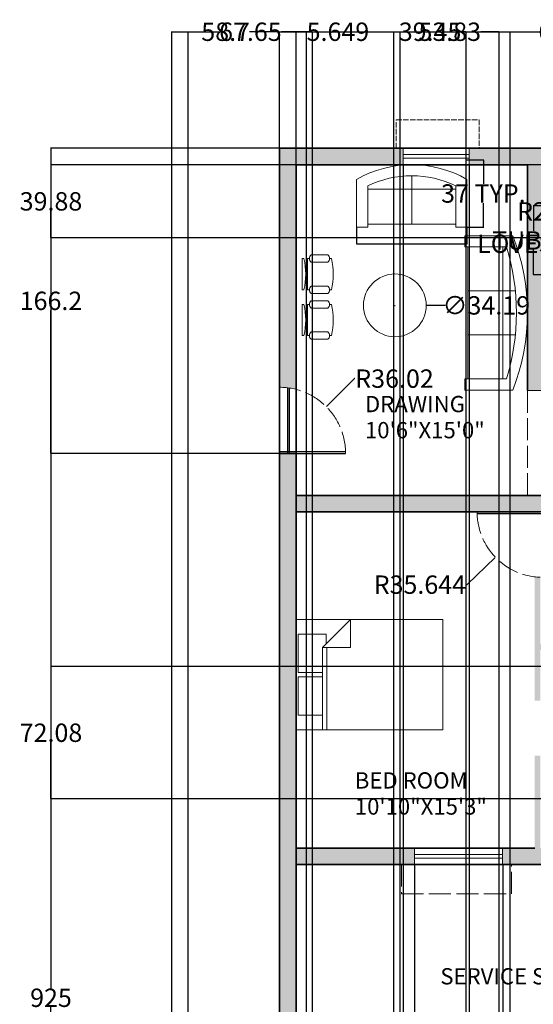
# Model space of a CAD drawing. Units: inches. Extents: x 300 to 1007, y 2 to 1069.
# Tile 8 of 12: x 337 to 617, y 533 to 1069. Entities that reach past the tile are written whole.
import ezdxf

# ---------------------------------------------------------------- set-up
doc = ezdxf.new("R2010")
doc.units = ezdxf.units.IN
doc.header["$MEASUREMENT"] = 0
doc.linetypes.add('ACAD_ISO02W100', pattern=[15, 12, -3])
for name, color, linetype, lineweight in [('A-ANNO-DIMS', 2, 'Continuous', 18), ('A-ANNO-TEXT', 7, 'Continuous', 18), ('A-AREA-IDEN', 7, 'Continuous', 18), ('A-DOOR', 3, 'Continuous', 25), ('A-DOOR-SWNG', 3, 'ACAD_ISO02W100', 13), ('A-FLOR-SLAB', 7, 'Continuous', 35), ('A-FURN', 8, 'Continuous', 18), ('A-GLAZ', 4, 'Continuous', 18), ('A-GLAZ-OVHD', 8, 'ACAD_ISO02W100', 13), ('A-WALL', 7, 'Continuous', 35), ('A-WALL-OVHD', 8, 'ACAD_ISO02W100', 18)]:
    doc.layers.add(name, color=color, linetype=linetype, lineweight=lineweight)
doc.layers.add('A-WALL-PATT', color=9, linetype='Continuous', lineweight=9, true_color=0xc7c8ca)
doc.styles.get("Standard").update_dxf_attribs({"font": 'arial.ttf'})
doc.dimstyles.get("Standard").update_dxf_attribs({"dimtxt": 10, "dimasz": 0.18, "dimexe": 0.18, "dimexo": 0.0625, "dimgap": 0.09, "dimtad": 0, "dimtih": 1, "dimtoh": 1, "dimdec": 0, "dimzin": 0, "dimdsep": 46, "dimlunit": 3, "dimtxsty": 'Standard', "dimcen": 0.09, "dimadec": 0, "dimazin": 0, "dimtfac": 1, "dimtdec": 0, "dimtofl": 0, "dimtmove": 0, "dimatfit": 3, "dimfxl": 1, "dimtolj": 1, "dimtzin": 0, "dimarcsym": 0})

# ---------------------------------------------------------------- blocks, each defined once
blk = doc.blocks.new('Chair - Desk')
for p, q in [((-8.5, 0), (-8.5, -1)), ((-8.5, 0), (8.5, 0)), ((8.5, 0), (8.5, -1)), ((-10.5, -5), (-10.5, -14)), ((-8.5, -3), (-8.5, -4)), ((-8.5, -3), (8.5, -3)), ((-6.5, -14), (-6.5, -5)), ((-2, -3), (-2, -1.9355)), ((2, -1.9576), (2, -3)), ((6.5, -5), (6.5, -14)), ((8.5, -3), (8.5, -4)), ((10.5, -14), (10.5, -5)), ((-8.5, -15), (-8.5, -16)), ((8.5, -15), (8.5, -16))]:
    blk.add_line(p, q)
for centre, radius, start, end in [((-8.5, -6.5), 2.5, 36.8699, 143.1301), ((0, 34.625), 36.625, 256.5803, 283.4197), ((8.5, -6.5), 2.5, 36.8699, 143.1301), ((-8.5, -12.5), 2.5, 216.8699, 323.1301), ((0, 19.625), 36.625, 256.5803, 283.4197), ((8.5, -12.5), 2.5, 216.8699, 323.1301)]:
    blk.add_arc(centre, radius, start, end)
blk = doc.blocks.new('Sofa - Roundback 7 ft.')
for p, q in [((-12.00002, -32.4421), (-12.00003, -6.5971)), ((11.99997, -32.4421), (11.99998, -6.5971)), ((-36.000027, -34), (-36.000027, -11.4696)), ((-35.999844, -13.3819), (35.9998, -13.3819)), ((35.99998, -34), (35.99998, -11.4696)), ((-36.000027, -32.4421), (35.99998, -32.4421))]:
    blk.add_line(p, q)
for points in [[(-36.000027, -34), (-42.000027, -34), (-42.000027, -8)], [(41.99998, -8), (41.99998, -34), (35.99998, -34)]]:
    blk.add_lwpolyline(points)
for centre, radius, start, end in [((0, -114.25), 114.25, 68.43141, 111.5686), ((-0.00001, -127.1968), 121.1968, 72.72033, 107.2797)]:
    blk.add_arc(centre, radius, start, end)
blk = doc.blocks.new('Sofa - Roundback Loveseat 5 ft.')
for p, q in [((0, -32.44198), (0, -5.99998)), ((-24, -33.99998), (-24, -11.46958)), ((-23.9998, -13.38178), (23.99986, -13.38178)), ((24.00004, -33.99998), (24.00004, -11.46958)), ((-24, -32.44198), (24.00004, -32.44198))]:
    blk.add_line(p, q)
for points in [[(-24, -33.99998), (-30, -33.99998), (-30, -7.99998)], [(30.00004, -7.99998), (30.00004, -33.99998), (24.00004, -33.99998)]]:
    blk.add_lwpolyline(points)
for centre, radius, start, end in [((0, -60.24998), 60.24998, 60.13715, 119.8628), ((0, -61.38438), 55.38444, 64.32083, 115.6792)]:
    blk.add_arc(centre, radius, start, end)
blk = doc.blocks.new('Bed - Queen')
for p, q in [((0, -80.00003), (0, 0)), ((0, 0), (59.99999, 0)), ((59.99999, 0), (59.99999, -80.00003)), ((7.99999, -1.2), (28.79998, -1.2)), ((7.99999, -14.4), (7.99999, -1.2)), ((28.79998, -1.2), (28.79998, -14.4)), ((31.19999, -1.2), (51.99999, -1.2)), ((31.19999, -14.4), (31.19999, -1.2)), ((51.99999, -1.2), (51.99999, -16.4)), ((0, -14.4), (44.8, -14.4)), ((59.99999, -29.6), (44.8, -14.4)), ((44.8, -14.4), (44.8, -29.6)), ((44.8, -16.8), (0, -16.8)), ((51.99999, -16.4), (46.79936, -16.4)), ((44.8, -29.6), (59.99999, -29.6)), ((59.99999, -80.00003), (0, -80.00003))]:
    blk.add_line(p, q)
blk = doc.blocks.new('WIN-48')
for p, q in [((-47.83, 0), (-47.83, 4.5)), ((-47.83, 4.5), (-47.83, -4.5)), ((0, 1), (-47.83, 1)), ((0, 4.5), (0, -4.5)), ((0, -1), (-47.83, -1))]:
    blk.add_line(p, q)
blk = doc.blocks.new('WIN-36')
for p, q in [((-36, -4.5), (-36, 4.5)), ((0, 1), (-36, 1)), ((-36, 0), (-36, -4.5)), ((0, -4.5), (0, 4.5)), ((0, -1), (-36, -1))]:
    blk.add_line(p, q)
blk = doc.blocks.new('WINDOW-HOOD-45')
at = {"ltscale": 0.25}
for p, q in [((0, 0), (0, 15.48)), ((0, 15.48), (45.18, 15.48)), ((45.18, 15.48), (45.18, 0))]:
    blk.add_line(p, q, dxfattribs=at)
blk = doc.blocks.new('*D39')
at = {"layer": 'A-ANNO-DIMS', "color": 0, "lineweight": -2, "transparency": 16777216}
for p, q in [((622.76, 968.04), (617.01, 968.04)), ((617.19, 967.86), (617.19, 954.44)), ((617.19, 930.63), (617.19, 944.04)), ((622.76, 930.45), (617.01, 930.45))]:
    blk.add_line(p, q, dxfattribs=at)
at = {"layer": 'A-ANNO-DIMS', "color": 0, "transparency": 16777216}
for points in [[(617.16, 967.86), (617.22, 967.86), (617.19, 968.04)], [(617.16, 930.63), (617.22, 930.63), (617.19, 930.45)]]:
    blk.add_solid(points, dxfattribs=at)
at = {"layer": 'Defpoints', "color": 0, "transparency": 16777216}
for p in [(622.83, 968.04), (617.19, 930.45), (622.83, 930.45)]:
    blk.add_point(p, dxfattribs=at)
at = {"layer": 'A-ANNO-DIMS', "color": 0, "transparency": 16777216, "insert": (617.19, 949.24), "char_height": 10, "attachment_point": 5}
blk.add_mtext('\\A1;TUB 38', dxfattribs=at)
blk = doc.blocks.new('*D49')
at = {"layer": 'A-ANNO-DIMS', "color": 0, "lineweight": -2, "transparency": 16777216}
for p, q in [((520.83, 956.38), (520.83, 947.27)), ((580.83, 956.38), (580.83, 947.27)), ((521.01, 947.45), (580.65, 947.45)), ((580.83, 947.45), (581.01, 947.45))]:
    blk.add_line(p, q, dxfattribs=at)
at = {"layer": 'A-ANNO-DIMS', "color": 0, "transparency": 16777216}
for points in [[(521.01, 947.48), (521.01, 947.42), (520.83, 947.45)], [(580.65, 947.48), (580.65, 947.42), (580.83, 947.45)]]:
    blk.add_solid(points, dxfattribs=at)
at = {"layer": 'Defpoints', "color": 0, "transparency": 16777216}
for p in [(520.83, 956.45), (580.83, 956.45), (580.83, 947.45)]:
    blk.add_point(p, dxfattribs=at)
at = {"layer": 'A-ANNO-DIMS', "color": 0, "transparency": 16777216, "insert": (644.03, 947.45), "char_height": 10, "attachment_point": 5}
blk.add_mtext('\\A1;LOVESEAT 60 TYP.', dxfattribs=at)
blk = doc.blocks.new('*D50')
at = {"layer": 'A-ANNO-DIMS', "color": 0, "lineweight": -2, "transparency": 16777216}
for p, q in [((580.89, 993.11), (590.01, 993.11)), ((589.83, 992.93), (589.83, 979.98)), ((589.83, 956.63), (589.83, 969.58)), ((580.89, 956.45), (590.01, 956.45))]:
    blk.add_line(p, q, dxfattribs=at)
at = {"layer": 'A-ANNO-DIMS', "color": 0, "transparency": 16777216}
for points in [[(589.8, 992.93), (589.86, 992.93), (589.83, 993.11)], [(589.8, 956.63), (589.86, 956.63), (589.83, 956.45)]]:
    blk.add_solid(points, dxfattribs=at)
at = {"layer": 'Defpoints', "color": 0, "transparency": 16777216}
for p in [(580.83, 993.11), (589.83, 993.11), (580.83, 956.45)]:
    blk.add_point(p, dxfattribs=at)
at = {"layer": 'A-ANNO-DIMS', "color": 0, "transparency": 16777216, "insert": (589.83, 974.78), "char_height": 10, "attachment_point": 5}
blk.add_mtext('\\A1;37 TYP.', dxfattribs=at)
blk = doc.blocks.new('*D74')
at = {"layer": 'A-ANNO-DIMS', "color": 0, "lineweight": -2, "transparency": 16777216}
for p, q in [((478.76, 999.45), (354.19, 999.45)), ((354.37, 999.27), (354.37, 542.11)), ((354.37, 74.56), (354.37, 531.72)), ((420.06, 74.38), (354.19, 74.38))]:
    blk.add_line(p, q, dxfattribs=at)
at = {"layer": 'A-ANNO-DIMS', "color": 0, "transparency": 16777216}
for points in [[(354.34, 999.27), (354.4, 999.27), (354.37, 999.45)], [(354.34, 74.56), (354.4, 74.56), (354.37, 74.38)]]:
    blk.add_solid(points, dxfattribs=at)
at = {"layer": 'Defpoints', "color": 0, "transparency": 16777216}
for p in [(354.37, 999.45), (478.83, 999.45), (420.12, 74.38)]:
    blk.add_point(p, dxfattribs=at)
at = {"layer": 'A-ANNO-DIMS', "color": 0, "transparency": 16777216, "insert": (354.37, 536.92), "char_height": 10, "attachment_point": 5}
blk.add_mtext('\\A1;925', dxfattribs=at)
blk = doc.blocks.new('*D75')
at = {"layer": 'A-ANNO-DIMS', "color": 0, "lineweight": -2, "transparency": 16777216}
for p, q in [((478.83, 999.51), (478.83, 1063.03)), ((479.01, 1062.85), (653.74, 1062.85)), ((850.65, 1062.85), (675.91, 1062.85)), ((850.83, 999.51), (850.83, 1063.03))]:
    blk.add_line(p, q, dxfattribs=at)
at = {"layer": 'A-ANNO-DIMS', "color": 0, "transparency": 16777216}
for points in [[(479.01, 1062.88), (479.01, 1062.82), (478.83, 1062.85)], [(850.65, 1062.88), (850.65, 1062.82), (850.83, 1062.85)]]:
    blk.add_solid(points, dxfattribs=at)
at = {"layer": 'Defpoints', "color": 0, "transparency": 16777216}
for p in [(850.83, 1062.85), (478.83, 999.45), (850.83, 999.45)]:
    blk.add_point(p, dxfattribs=at)
at = {"layer": 'A-ANNO-DIMS', "color": 0, "transparency": 16777216, "insert": (664.83, 1062.85), "char_height": 10, "attachment_point": 5}
blk.add_mtext('\\A1;372', dxfattribs=at)
blk = doc.blocks.new('*D79')
at = {"layer": 'A-ANNO-DIMS', "color": 0, "lineweight": -2, "transparency": 16777216}
for p, q in [((420.12, 482.45), (420.12, 1063.03)), ((420.3, 1062.85), (436.4, 1062.85)), ((478.65, 1062.85), (462.55, 1062.85)), ((478.83, 482.45), (478.83, 1063.03))]:
    blk.add_line(p, q, dxfattribs=at)
at = {"layer": 'A-ANNO-DIMS', "color": 0, "transparency": 16777216}
for points in [[(420.3, 1062.88), (420.3, 1062.82), (420.12, 1062.85)], [(478.65, 1062.88), (478.65, 1062.82), (478.83, 1062.85)]]:
    blk.add_solid(points, dxfattribs=at)
at = {"layer": 'Defpoints', "color": 0, "transparency": 16777216}
for p in [(478.83, 1062.85), (420.12, 482.38), (478.83, 482.38)]:
    blk.add_point(p, dxfattribs=at)
at = {"layer": 'A-ANNO-DIMS', "color": 0, "transparency": 16777216, "insert": (449.47, 1062.85), "char_height": 10, "attachment_point": 5}
blk.add_mtext('\\A1;58.7', dxfattribs=at)
blk = doc.blocks.new('*D81')
at = {"layer": 'A-ANNO-DIMS', "color": 0, "lineweight": -2, "transparency": 16777216}
for p, q in [((705.53, 717.25), (354.19, 717.25)), ((354.37, 717.07), (354.37, 686.41)), ((354.37, 645.35), (354.37, 676.01)), ((705.53, 645.17), (354.19, 645.17))]:
    blk.add_line(p, q, dxfattribs=at)
at = {"layer": 'A-ANNO-DIMS', "color": 0, "transparency": 16777216}
for points in [[(354.34, 717.07), (354.4, 717.07), (354.37, 717.25)], [(354.34, 645.35), (354.4, 645.35), (354.37, 645.17)]]:
    blk.add_solid(points, dxfattribs=at)
at = {"layer": 'Defpoints', "color": 0, "transparency": 16777216}
for p in [(354.37, 717.25), (705.59, 717.25), (705.59, 645.17)]:
    blk.add_point(p, dxfattribs=at)
at = {"layer": 'A-ANNO-DIMS', "color": 0, "transparency": 16777216, "insert": (354.37, 681.21), "char_height": 10, "attachment_point": 5}
blk.add_mtext('\\A1;72.08', dxfattribs=at)
blk = doc.blocks.new('*D88')
at = {"layer": 'A-ANNO-DIMS', "color": 0, "lineweight": -2, "transparency": 16777216}
for p, q in [((429.12, 83.45), (429.12, 1063.03)), ((429.3, 1062.85), (445.92, 1062.85)), ((496.59, 1062.85), (479.97, 1062.85)), ((496.77, 83.45), (496.77, 1063.03))]:
    blk.add_line(p, q, dxfattribs=at)
at = {"layer": 'A-ANNO-DIMS', "color": 0, "transparency": 16777216}
for points in [[(429.3, 1062.88), (429.3, 1062.82), (429.12, 1062.85)], [(496.59, 1062.88), (496.59, 1062.82), (496.77, 1062.85)]]:
    blk.add_solid(points, dxfattribs=at)
at = {"layer": 'Defpoints', "color": 0, "transparency": 16777216}
for p in [(496.77, 1062.85), (429.12, 83.38), (496.77, 83.38)]:
    blk.add_point(p, dxfattribs=at)
at = {"layer": 'A-ANNO-DIMS', "color": 0, "transparency": 16777216, "insert": (462.95, 1062.85), "char_height": 10, "attachment_point": 5}
blk.add_mtext('\\A1;67.65', dxfattribs=at)
blk = doc.blocks.new('*D89')
at = {"layer": 'A-ANNO-DIMS', "color": 0, "lineweight": -2, "transparency": 16777216}
for p, q in [((544.6, 83.45), (544.6, 1063.03)), ((544.78, 1062.85), (554.56, 1062.85)), ((598.25, 1062.85), (588.48, 1062.85)), ((598.43, 83.45), (598.43, 1063.03))]:
    blk.add_line(p, q, dxfattribs=at)
at = {"layer": 'A-ANNO-DIMS', "color": 0, "transparency": 16777216}
for points in [[(544.78, 1062.88), (544.78, 1062.82), (544.6, 1062.85)], [(598.25, 1062.88), (598.25, 1062.82), (598.43, 1062.85)]]:
    blk.add_solid(points, dxfattribs=at)
at = {"layer": 'Defpoints', "color": 0, "transparency": 16777216}
for p in [(598.43, 1062.85), (544.6, 83.38), (598.43, 83.38)]:
    blk.add_point(p, dxfattribs=at)
at = {"layer": 'A-ANNO-DIMS', "color": 0, "transparency": 16777216, "insert": (571.52, 1062.85), "char_height": 10, "attachment_point": 5}
blk.add_mtext('\\A1;53.83', dxfattribs=at)
blk = doc.blocks.new('*D93')
at = {"layer": 'A-ANNO-DIMS', "color": 0, "lineweight": -2, "transparency": 16777216}
for p, q in [((478.76, 999.45), (354.19, 999.45)), ((354.37, 999.27), (354.37, 921.55)), ((354.37, 833.44), (354.37, 911.16)), ((478.76, 833.26), (354.19, 833.26))]:
    blk.add_line(p, q, dxfattribs=at)
at = {"layer": 'A-ANNO-DIMS', "color": 0, "transparency": 16777216}
for points in [[(354.34, 999.27), (354.4, 999.27), (354.37, 999.45)], [(354.34, 833.44), (354.4, 833.44), (354.37, 833.26)]]:
    blk.add_solid(points, dxfattribs=at)
at = {"layer": 'Defpoints', "color": 0, "transparency": 16777216}
for p in [(354.37, 999.45), (478.83, 999.45), (478.83, 833.26)]:
    blk.add_point(p, dxfattribs=at)
at = {"layer": 'A-ANNO-DIMS', "color": 0, "transparency": 16777216, "insert": (354.37, 916.35), "char_height": 10, "attachment_point": 5}
blk.add_mtext('\\A1;166.2', dxfattribs=at)
blk = doc.blocks.new('*D94')
at = {"layer": 'A-ANNO-DIMS', "color": 0, "lineweight": -2, "transparency": 16777216}
for p, q in [((841.76, 990.45), (354.19, 990.45)), ((354.37, 990.27), (354.37, 975.71)), ((354.37, 950.75), (354.37, 965.31)), ((841.76, 950.57), (354.19, 950.57))]:
    blk.add_line(p, q, dxfattribs=at)
at = {"layer": 'A-ANNO-DIMS', "color": 0, "transparency": 16777216}
for points in [[(354.34, 990.27), (354.4, 990.27), (354.37, 990.45)], [(354.34, 950.75), (354.4, 950.75), (354.37, 950.57)]]:
    blk.add_solid(points, dxfattribs=at)
at = {"layer": 'Defpoints', "color": 0, "transparency": 16777216}
for p in [(354.37, 990.45), (841.83, 990.45), (841.83, 950.57)]:
    blk.add_point(p, dxfattribs=at)
at = {"layer": 'A-ANNO-DIMS', "color": 0, "transparency": 16777216, "insert": (354.37, 970.51), "char_height": 10, "attachment_point": 5}
blk.add_mtext('\\A1;39.88', dxfattribs=at)
blk = doc.blocks.new('*D97')
at = {"layer": 'A-ANNO-DIMS', "color": 0, "lineweight": -2, "transparency": 16777216}
for p, q in [((487.83, 482.45), (487.83, 1063.03)), ((488.01, 1062.85), (493.3, 1062.85)), ((493.48, 482.45), (493.48, 1063.03)), ((493.48, 1062.85), (493.66, 1062.85))]:
    blk.add_line(p, q, dxfattribs=at)
at = {"layer": 'A-ANNO-DIMS', "color": 0, "transparency": 16777216}
for points in [[(488.01, 1062.88), (488.01, 1062.82), (487.83, 1062.85)], [(493.3, 1062.88), (493.3, 1062.82), (493.48, 1062.85)]]:
    blk.add_solid(points, dxfattribs=at)
at = {"layer": 'Defpoints', "color": 0, "transparency": 16777216}
for p in [(493.48, 1062.85), (487.83, 482.38), (493.48, 482.38)]:
    blk.add_point(p, dxfattribs=at)
at = {"layer": 'A-ANNO-DIMS', "color": 0, "transparency": 16777216, "insert": (510.63, 1062.85), "char_height": 10, "attachment_point": 5}
blk.add_mtext('\\A1;5.649', dxfattribs=at)
blk = doc.blocks.new('*D98')
at = {"layer": 'A-ANNO-DIMS', "color": 0, "lineweight": -2, "transparency": 16777216}
for p, q in [((541.08, 482.45), (541.08, 1063.03)), ((541.26, 1062.85), (543.81, 1062.85)), ((580.35, 1062.85), (577.8, 1062.85)), ((580.53, 482.45), (580.53, 1063.03))]:
    blk.add_line(p, q, dxfattribs=at)
at = {"layer": 'A-ANNO-DIMS', "color": 0, "transparency": 16777216}
for points in [[(541.26, 1062.88), (541.26, 1062.82), (541.08, 1062.85)], [(580.35, 1062.88), (580.35, 1062.82), (580.53, 1062.85)]]:
    blk.add_solid(points, dxfattribs=at)
at = {"layer": 'Defpoints', "color": 0, "transparency": 16777216}
for p in [(580.53, 1062.85), (541.08, 482.38), (580.53, 482.38)]:
    blk.add_point(p, dxfattribs=at)
at = {"layer": 'A-ANNO-DIMS', "color": 0, "transparency": 16777216, "insert": (560.81, 1062.85), "char_height": 10, "attachment_point": 5}
blk.add_mtext('\\A1;39.45', dxfattribs=at)
blk = doc.blocks.new('*D99')
at = {"layer": 'A-ANNO-DIMS', "color": 0, "lineweight": -2, "transparency": 16777216}
for p, q in [((604.49, 482.45), (604.49, 1063.03)), ((604.67, 1062.85), (619.83, 1062.85)), ((668.97, 1062.85), (653.8, 1062.85)), ((669.15, 482.45), (669.15, 1063.03))]:
    blk.add_line(p, q, dxfattribs=at)
at = {"layer": 'A-ANNO-DIMS', "color": 0, "transparency": 16777216}
for points in [[(604.67, 1062.88), (604.67, 1062.82), (604.49, 1062.85)], [(668.97, 1062.88), (668.97, 1062.82), (669.15, 1062.85)]]:
    blk.add_solid(points, dxfattribs=at)
at = {"layer": 'Defpoints', "color": 0, "transparency": 16777216}
for p in [(669.15, 1062.85), (604.49, 482.38), (669.15, 482.38)]:
    blk.add_point(p, dxfattribs=at)
at = {"layer": 'A-ANNO-DIMS', "color": 0, "transparency": 16777216, "insert": (636.82, 1062.85), "char_height": 10, "attachment_point": 5}
blk.add_mtext('\\A1;64.66', dxfattribs=at)
blk = doc.blocks.new('*D101')
at = {"layer": 'A-ANNO-DIMS', "color": 0, "lineweight": -2, "transparency": 16777216}
for p, q in [((487.83, 609.38), (487.83, 8.45)), ((552.34, 609.38), (552.34, 8.45)), ((488.01, 8.63), (504.06, 8.63)), ((552.16, 8.63), (536.11, 8.63))]:
    blk.add_line(p, q, dxfattribs=at)
at = {"layer": 'A-ANNO-DIMS', "color": 0, "transparency": 16777216}
for points in [[(488.01, 8.66), (488.01, 8.6), (487.83, 8.63)], [(552.16, 8.66), (552.16, 8.6), (552.34, 8.63)]]:
    blk.add_solid(points, dxfattribs=at)
at = {"layer": 'Defpoints', "color": 0, "transparency": 16777216}
for p in [(487.83, 609.45), (552.34, 609.45), (552.34, 8.63)]:
    blk.add_point(p, dxfattribs=at)
at = {"layer": 'A-ANNO-DIMS', "color": 0, "transparency": 16777216, "insert": (520.08, 8.63), "char_height": 10, "attachment_point": 5}
blk.add_mtext('\\A1;64.51', dxfattribs=at)
blk = doc.blocks.new('*D102')
at = {"layer": 'A-ANNO-DIMS', "color": 0, "lineweight": -2, "transparency": 16777216}
for p, q in [((600.34, 609.38), (600.34, 8.45)), ((652.99, 609.38), (652.99, 8.45)), ((600.52, 8.63), (609.71, 8.63)), ((652.81, 8.63), (643.62, 8.63))]:
    blk.add_line(p, q, dxfattribs=at)
at = {"layer": 'A-ANNO-DIMS', "color": 0, "transparency": 16777216}
for points in [[(600.52, 8.66), (600.52, 8.6), (600.34, 8.63)], [(652.81, 8.66), (652.81, 8.6), (652.99, 8.63)]]:
    blk.add_solid(points, dxfattribs=at)
at = {"layer": 'Defpoints', "color": 0, "transparency": 16777216}
for p in [(600.34, 609.45), (652.99, 609.45), (652.99, 8.63)]:
    blk.add_point(p, dxfattribs=at)
at = {"layer": 'A-ANNO-DIMS', "color": 0, "transparency": 16777216, "insert": (626.66, 8.63), "char_height": 10, "attachment_point": 5}
blk.add_mtext('\\A1;52.66', dxfattribs=at)
blk = doc.blocks.new('*D105')
at = {"layer": 'A-ANNO-DIMS', "color": 0, "lineweight": -2, "transparency": 16777216}
for p, q in [((487.83, 990.38), (487.83, 8.45)), ((546.1, 990.38), (546.1, 8.45)), ((488.01, 8.63), (499.99, 8.63)), ((545.92, 8.63), (533.94, 8.63))]:
    blk.add_line(p, q, dxfattribs=at)
at = {"layer": 'A-ANNO-DIMS', "color": 0, "transparency": 16777216}
for points in [[(488.01, 8.66), (488.01, 8.6), (487.83, 8.63)], [(545.92, 8.66), (545.92, 8.6), (546.1, 8.63)]]:
    blk.add_solid(points, dxfattribs=at)
at = {"layer": 'Defpoints', "color": 0, "transparency": 16777216}
for p in [(487.83, 990.45), (546.1, 990.45), (546.1, 8.63)]:
    blk.add_point(p, dxfattribs=at)
at = {"layer": 'A-ANNO-DIMS', "color": 0, "transparency": 16777216, "insert": (516.97, 8.63), "char_height": 10, "attachment_point": 5}
blk.add_mtext('\\A1;58.28', dxfattribs=at)
blk = doc.blocks.new('*D106')
at = {"layer": 'A-ANNO-DIMS', "color": 0, "lineweight": -2, "transparency": 16777216}
for p, q in [((582.11, 990.38), (582.11, 8.45)), ((630.49, 990.38), (630.49, 8.45)), ((582.29, 8.63), (589.12, 8.63)), ((630.31, 8.63), (623.47, 8.63))]:
    blk.add_line(p, q, dxfattribs=at)
at = {"layer": 'A-ANNO-DIMS', "color": 0, "transparency": 16777216}
for points in [[(582.29, 8.66), (582.29, 8.6), (582.11, 8.63)], [(630.31, 8.66), (630.31, 8.6), (630.49, 8.63)]]:
    blk.add_solid(points, dxfattribs=at)
at = {"layer": 'Defpoints', "color": 0, "transparency": 16777216}
for p in [(582.11, 990.45), (630.49, 990.45), (630.49, 8.63)]:
    blk.add_point(p, dxfattribs=at)
at = {"layer": 'A-ANNO-DIMS', "color": 0, "transparency": 16777216, "insert": (606.3, 8.63), "char_height": 10, "attachment_point": 5}
blk.add_mtext('\\A1;48.38', dxfattribs=at)
blk = doc.blocks.new('*D110')
at = {"layer": 'A-ANNO-DIMS', "color": 0, "lineweight": -2, "transparency": 16777216}
for p, q in [((541.56, 913.87), (541.74, 913.87)), ((541.65, 913.78), (541.65, 913.96)), ((569, 913.87), (558.92, 913.87))]:
    blk.add_line(p, q, dxfattribs=at)
at = {"layer": 'A-ANNO-DIMS', "color": 0, "transparency": 16777216}
blk.add_solid([(558.92, 913.9), (558.92, 913.84), (558.74, 913.87)], dxfattribs=at)
at = {"layer": 'Defpoints', "color": 0, "transparency": 16777216}
for p in [(524.55, 913.87), (558.74, 913.87)]:
    blk.add_point(p, dxfattribs=at)
at = {"layer": 'A-ANNO-DIMS', "color": 0, "transparency": 16777216, "insert": (591.41, 913.87), "char_height": 10, "attachment_point": 5}
blk.add_mtext('\\A1;∅34.19', dxfattribs=at)
blk = doc.blocks.new('*D112')
at = {"layer": 'A-ANNO-DIMS', "color": 0, "lineweight": -2, "transparency": 16777216}
for p, q in [((519.57, 874), (504.41, 858.85)), ((519.75, 874), (519.57, 874)), ((478.72, 833.26), (478.9, 833.26)), ((478.81, 833.17), (478.81, 833.35))]:
    blk.add_line(p, q, dxfattribs=at)
at = {"layer": 'A-ANNO-DIMS', "color": 0, "transparency": 16777216}
blk.add_solid([(504.39, 858.87), (504.43, 858.83), (504.28, 858.72)], dxfattribs=at)
at = {"layer": 'Defpoints', "color": 0, "transparency": 16777216}
for p in [(504.28, 858.72), (478.81, 833.26)]:
    blk.add_point(p, dxfattribs=at)
at = {"layer": 'A-ANNO-DIMS', "color": 0, "transparency": 16777216, "insert": (541.44, 874), "char_height": 10, "attachment_point": 5}
blk.add_mtext('\\A1;R36.02', dxfattribs=at)
blk = doc.blocks.new('*D113')
at = {"layer": 'A-ANNO-DIMS', "color": 0, "lineweight": -2, "transparency": 16777216}
for p, q in [((621.98, 801.45), (622.16, 801.45)), ((622.07, 801.36), (622.07, 801.54)), ((581.05, 761.83), (596.3, 776.56)), ((580.87, 761.83), (581.05, 761.83))]:
    blk.add_line(p, q, dxfattribs=at)
at = {"layer": 'A-ANNO-DIMS', "color": 0, "transparency": 16777216}
blk.add_solid([(596.28, 776.58), (596.32, 776.54), (596.43, 776.68)], dxfattribs=at)
at = {"layer": 'Defpoints', "color": 0, "transparency": 16777216}
for p in [(622.07, 801.45), (596.43, 776.68)]:
    blk.add_point(p, dxfattribs=at)
at = {"layer": 'A-ANNO-DIMS', "color": 0, "transparency": 16777216, "insert": (555.25, 761.83), "char_height": 10, "attachment_point": 5}
blk.add_mtext('\\A1;R35.644', dxfattribs=at)
blk = doc.blocks.new('*D118')
at = {"layer": 'A-ANNO-DIMS', "color": 0, "lineweight": -2, "transparency": 16777216}
for p, q in [((651.31, 965.03), (651.49, 965.03)), ((651.49, 965.03), (663.55, 952.19)), ((683.9, 930.45), (684.08, 930.45)), ((683.99, 930.36), (683.99, 930.54))]:
    blk.add_line(p, q, dxfattribs=at)
at = {"layer": 'A-ANNO-DIMS', "color": 0, "transparency": 16777216}
blk.add_solid([(663.57, 952.21), (663.53, 952.17), (663.68, 952.06)], dxfattribs=at)
at = {"layer": 'Defpoints', "color": 0, "transparency": 16777216}
for p in [(663.68, 952.06), (683.99, 930.45)]:
    blk.add_point(p, dxfattribs=at)
at = {"layer": 'A-ANNO-DIMS', "color": 0, "transparency": 16777216, "insert": (629.57, 965.03), "char_height": 10, "attachment_point": 5}
blk.add_mtext('\\A1;R29.66', dxfattribs=at)

msp = doc.modelspace()

# ---------------------------------------------------------------- hatches: boundary and pattern name
at = {"layer": 'A-WALL-PATT'}
h = msp.add_hatch(color=256, dxfattribs=at)
h.dxf.hatch_style = 1
h.paths.add_polyline_path([(546.104, 999.4468), (478.8267, 999.4468), (478.8267, 869.2798, -0.06322715), (487.8267, 868.1328), (487.8267, 990.4468), (546.104, 990.4468)])
h.paths.add_polyline_path([(630.4852, 999.4468), (582.106, 999.4468), (582.106, 990.4468), (613.8267, 990.4468), (613.8267, 867.4468), (622.8267, 867.4468), (622.8267, 990.4468), (630.4852, 990.4468)])
h.paths.add_polyline_path([(702.0883, 999.4468), (650.4653, 999.4468), (650.4653, 990.4468), (682.8267, 990.4468), (682.8267, 960.0824, -0.02530575), (685.8267, 960.0478), (685.8267, 990.4468), (702.0883, 990.4468)])
h.paths.add_polyline_path([(850.8267, 999.4468), (737.5888, 999.4468), (737.5888, 990.4468), (841.8267, 990.4468), (841.8267, 950.5685), (850.8267, 950.5685)])
h.paths.add_polyline_path([(685.8267, 930.4465), (682.8267, 930.4465), (682.8267, 888.4468), (682.8267, 867.4468), (685.8267, 867.4468), (697.4169, 867.4468), (697.4169, 870.4468), (685.8267, 870.4468), (685.8267, 888.4468)])
h.paths.add_polyline_path([(682.8267, 931.4465), (654.3436, 931.4465, 0.00843109), (654.3267, 930.4465), (682.8267, 930.4465)])
h.paths.add_polyline_path([(685.8267, 931.4465), (682.8267, 931.4465), (682.8267, 930.4465), (685.8267, 930.4465)])
h.paths.add_polyline_path([(682.8267, 888.4468), (622.8267, 888.4468), (622.8267, 885.4468), (682.8267, 885.4468)])
h.paths.add_polyline_path([(850.8267, 870.4468), (850.8267, 914.7851), (841.8267, 914.7851), (841.8267, 870.4468), (732.7101, 870.4468, -0.02120595), (732.8267, 867.4468), (779.8267, 867.4468), (779.8267, 749.4468), (782.8267, 749.4468), (788.8267, 749.4468), (788.8267, 861.4468), (841.8267, 861.4468), (841.8267, 749.4468), (850.8267, 749.4468)])
h.paths.add_polyline_path([(622.8267, 810.4468), (487.8267, 810.4468), (487.8267, 833.2626), (478.8267, 833.2626), (478.8267, 609.4468), (478.8267, 482.3847), (487.8267, 482.3847), (487.8267, 801.4468), (620.8267, 801.4468), (622.8267, 801.4468)])
h.paths.add_polyline_path([(680.8267, 729.4468), (620.8267, 729.4468), (620.8267, 765.8246, -0.02111352), (617.8267, 766.0562), (617.8267, 698.7303), (620.8267, 698.7303), (620.8267, 726.4468), (680.8267, 726.4468)])
h.paths.add_polyline_path([(620.8267, 668.8122, -0.02498293), (617.8267, 668.6448), (617.8267, 618.4468), (600.3357, 618.4468), (600.3357, 609.4468), (652.9929, 609.4468), (652.9929, 618.4468), (620.8267, 618.4468)])
h.paths.add_polyline_path([(552.3393, 618.4468), (487.8267, 618.4468), (487.8267, 609.4468), (552.3393, 609.4468)], flags=17)
h.paths.add_polyline_path([(694.5763, 618.4468), (683.8267, 618.4468), (683.8267, 726.4468), (683.8267, 749.4468), (680.8267, 749.4468), (680.8267, 740.4468), (680.8267, 726.4468), (680.8267, 618.4468), (674.1573, 618.4468), (674.1573, 609.4468), (680.8267, 609.4468), (694.5763, 609.4468)])
h.paths.add_polyline_path([(850.8267, 642.8902), (841.8267, 642.8902), (841.8267, 618.4468), (782.8267, 618.4468), (782.8267, 708.0513, -0.02308839), (779.8267, 707.9092), (779.8267, 618.4468), (730.1068, 618.4468), (730.1068, 609.4468), (779.8267, 609.4468), (841.8267, 609.4468), (841.8267, 482.3847), (850.8267, 482.3847)])
h.paths.add_polyline_path([(850.8267, 749.4468), (841.8267, 749.4468), (841.8267, 705.9119), (850.8267, 705.9119)])
h.paths.add_polyline_path([(841.8267, 749.4468), (782.8267, 749.4468), (779.8267, 749.4468), (761.9959, 749.4468), (761.9959, 740.4468), (779.8267, 740.4468), (812.3267, 740.4468), (841.8267, 740.4468)])
h.paths.add_polyline_path([(669.1457, 482.3847), (604.489, 482.3847), (604.489, 473.3847), (631.1217, 473.3847), (631.1217, 436.0244, -0.02504709), (634.1217, 436.1748), (634.1217, 436.4367), (634.1217, 473.3847), (669.1457, 473.3847)], flags=17)
h.paths.add_polyline_path([(580.5305, 482.3847), (571.1217, 482.3847), (541.0813, 482.3847), (541.0813, 473.3847), (562.1217, 473.3847), (562.1217, 326.3847), (571.1217, 326.3847), (571.1217, 362.3847), (631.1217, 362.3847), (631.1217, 326.3847), (706.9024, 326.3847, -0.02105388), (706.9999, 329.3847), (634.1217, 329.3847), (634.1217, 365.3847), (634.1217, 406.1748), (631.1217, 406.1748), (631.1217, 365.3847), (571.1217, 365.3847), (571.1217, 473.3847), (580.5305, 473.3847)])
h.paths.add_polyline_path([(493.4756, 482.3847), (420.1217, 482.3847), (420.1217, 445.3134), (429.1217, 445.3134), (429.1217, 473.3847), (493.4756, 473.3847)])
h.paths.add_polyline_path([(786.2236, 482.3847), (716.7793, 482.3847), (716.7793, 473.3847), (766.1217, 473.3847), (766.1217, 329.3847), (742.5583, 329.3847), (742.5583, 326.3847), (766.1217, 326.3847), (766.1217, 316.0647), (769.1217, 316.0647), (769.1217, 326.3847), (769.1217, 473.3847), (786.2236, 473.3847)])
h.paths.add_polyline_path([(910.1217, 482.3847), (822.7166, 482.3847), (822.7166, 473.3847), (901.1217, 473.3847), (901.1217, 402.5393), (910.1217, 402.5393)])
h.paths.add_polyline_path([(910.1217, 366.1034), (901.1217, 366.1034), (901.1217, 329.3847), (814.1217, 329.3847), (814.1217, 312.5176), (817.1217, 312.5176), (817.1217, 326.3847), (901.1217, 326.3847), (901.1217, 293.0319), (910.1217, 293.0319), (910.1217, 326.3847)])
h.paths.add_polyline_path([(910.1217, 268.9355), (901.1217, 268.9355), (901.1217, 254.3847), (817.1217, 254.3847), (817.1217, 290.5411, -0.03396715), (814.1217, 290.3847), (814.1217, 254.3847), (775.1217, 254.3847), (775.1217, 281.5164), (769.1217, 281.5164), (769.1217, 292.1577), (766.1217, 292.1577), (766.1217, 254.3847), (766.1217, 220.1938), (775.5079, 220.1938), (775.5079, 251.3847), (817.1217, 251.3847), (901.1217, 251.3847), (901.1217, 152.3847), (819.0246, 152.3847, -0.02493798), (818.9117, 149.3847), (901.1217, 149.3847), (901.1217, 92.3847), (901.1217, 83.3847), (874.3528, 83.3847), (874.3528, 74.3847), (910.1217, 74.3847), (910.1217, 92.3847), (910.1217, 149.3847)])
h.paths.add_polyline_path([(429.1217, 325.0924), (420.1217, 325.0924), (420.1217, 263.3847), (420.1217, 244.9834), (429.1217, 244.9834), (429.1217, 269.3847), (571.1217, 269.3847), (571.1217, 272.3847), (562.1217, 272.3847), (429.1217, 272.3847)])
h.paths.add_polyline_path([(429.1217, 208.998), (420.1217, 208.998), (420.1217, 74.3847), (496.7704, 74.3847), (496.7704, 83.3847), (429.1217, 83.3847)])
h.paths.add_polyline_path([(598.4322, 83.3847), (571.1217, 83.3847), (571.1217, 122.1171), (562.1217, 122.1171), (562.1217, 83.3847), (544.6031, 83.3847), (544.6031, 74.3847), (598.4322, 74.3847)])
h.paths.add_polyline_path([(797.0822, 83.3847), (769.1217, 83.3847), (769.1217, 149.3847), (788.9123, 149.3847), (788.9123, 152.3847), (769.1217, 152.3847), (769.1217, 178.0167), (766.1217, 178.0167), (766.1217, 152.3847), (735.3598, 152.3847), (735.3598, 143.3847), (766.1217, 143.3847), (766.1217, 83.3847), (634.1217, 83.3847), (634.1217, 143.3847), (659.7326, 143.3847), (659.7326, 152.3847), (634.1217, 152.3847), (634.1217, 194.3847), (571.1217, 194.3847), (571.1217, 233.7289, -0.06379947), (562.1217, 234.7942), (562.1217, 163.4485), (567.7403, 163.4485), (567.7403, 152.3847), (571.1217, 152.3847), (571.1217, 191.3847), (631.1217, 191.3847), (631.1217, 83.3847), (621.979, 83.3847), (621.979, 74.3847), (631.1217, 74.3847), (797.0822, 74.3847)])

# ---------------------------------------------------------------- linework, layer by layer
at = {"layer": 'A-DOOR'}
for p, q in [((478.8267, 833.2626), (478.8267, 869.2798)), ((483.3267, 833.2626), (483.3267, 868.9954)), ((484.3267, 833.2626), (484.3267, 868.8547)), ((478.8267, 834.2626), (514.8267, 834.2626)), ((487.8267, 833.2626), (478.8267, 833.2626)), ((478.8267, 833.2626), (514.8267, 833.2626)), ((622.8267, 801.4468), (586.4237, 801.4468)), ((622.8267, 800.4468), (586.4237, 800.4468))]:
    msp.add_line(p, q, dxfattribs=at)
at = {"layer": 'A-DOOR-SWNG'}
for centre, radius, start, end in [((478.8095, 833.2626), 36.0172, 0, 89.972576), ((622.0675, 801.4468), 35.6438, 180, 268.005096)]:
    msp.add_arc(centre, radius, start, end, dxfattribs=at)
at = {"layer": 'A-FLOR-SLAB'}
msp.add_line((478.8267, 482.3847), (478.8267, 609.4468), dxfattribs=at)
at = {"layer": 'A-FURN'}
msp.add_circle((541.6474, 913.868), 17.0937, dxfattribs=at)
at = {"layer": 'A-GLAZ-OVHD'}
for p, q in [((545.1625, 609.4468), (545.1625, 593.4374)), ((605.1509, 593.4374), (605.1509, 609.4468)), ((545.1625, 593.4374), (605.1509, 593.4374))]:
    msp.add_line(p, q, dxfattribs=at)
at = {"layer": 'A-WALL'}
for p, q in [((478.8267, 999.4468), (478.8267, 609.4468)), ((478.8267, 999.4468), (850.8267, 999.4468)), ((613.8267, 999.4468), (487.8267, 999.4468)), ((487.8267, 990.4468), (487.8267, 868.1328)), ((613.8267, 990.4468), (487.8267, 990.4468)), ((613.8267, 867.4468), (613.8267, 990.4468)), ((487.8267, 834.2626), (487.8267, 810.4468)), ((487.8267, 810.4468), (622.8267, 810.4468)), ((478.8267, 801.4468), (478.8267, 618.4468)), ((487.8267, 801.4468), (613.8267, 801.4468)), ((487.8267, 801.4468), (487.8267, 482.3847)), ((620.8267, 801.4468), (487.8267, 801.4468)), ((487.8267, 618.4468), (617.8267, 618.4468)), ((487.8267, 609.4468), (841.8267, 609.4468))]:
    msp.add_line(p, q, dxfattribs=at)
at = {"layer": 'A-WALL-OVHD'}
for p, q in [((622.8267, 867.4468), (613.8267, 867.4468)), ((613.8267, 867.4468), (613.8267, 810.4468))]:
    msp.add_line(p, q, dxfattribs=at)

# ---------------------------------------------------------------- block references
at = {"layer": 'A-FURN'}
msp.add_blockref('Sofa - Roundback Loveseat 5 ft.', (550.8267, 990.4468), dxfattribs=at)
for name, p, rotation in [('Sofa - Roundback 7 ft.', (613.8267, 909.7946), 270), ('Chair - Desk', (491.1113, 930.8509), 90), ('Chair - Desk', (491.1113, 905.9112), 90), ('Bed - Queen', (487.8267, 682.8033), 90)]:
    msp.add_blockref(name, p, dxfattribs=dict(at, rotation=rotation))
at = {"layer": 'A-GLAZ'}
msp.add_blockref('WIN-36', (582.106, 994.9468), dxfattribs=at)
at = {"layer": 'A-GLAZ', "xscale": 1.003421419532996}
msp.add_blockref('WIN-48', (600.3357, 613.9468), dxfattribs=at)
at = {"layer": 'A-GLAZ-OVHD'}
msp.add_blockref('WINDOW-HOOD-45', (542.3772, 999.4468), dxfattribs=at)

# ---------------------------------------------------------------- texts
at = {"layer": 'A-ANNO-TEXT'}
msp.add_text('SERVICE SLAB STIL COVERED SALB', height=8.843498, dxfattribs=at).set_placement((566.3949, 544.1919))
at = {"layer": 'A-AREA-IDEN'}
for s, height, p in [('DRAWING', 8.8435, (525.3459, 855.7291)), ('10\'6"X15\'0"', 8.843498, (525.3459, 841.5228)), ('BED ROOM', 8.8435, (519.8318, 650.8284)), ('10\'10"X15\'3"', 8.843498, (519.8318, 636.6221))]:
    msp.add_text(s, height=height, dxfattribs=at).set_placement(p)

# ---------------------------------------------------------------- dimensions: what is measured, and where the dimension line sits
at = {"layer": 'A-ANNO-DIMS'}
for base, p1, p2, override, picture, middle in [((478.8267, 1062.8469), (420.1217, 482.3847), (478.8267, 482.3847), {"dimdec": 1, "dimlfac": 1, "dimrnd": 0, "dimzin": 0, "dimdsep": 46, "dimlunit": 2}, '*D79', (449.4742, 1062.8469)), ((496.7704, 1062.8469), (429.1217, 83.3847), (496.7704, 83.3847), {"dimdec": 2, "dimlfac": 1, "dimrnd": 0, "dimzin": 0, "dimdsep": 46, "dimlunit": 2}, '*D88', (462.946, 1062.8469)), ((850.8267, 1062.8469), (478.8267, 999.4468), (850.8267, 999.4468), {"dimdec": 0, "dimlfac": 1, "dimrnd": 0, "dimzin": 0, "dimdsep": 46, "dimlunit": 2}, '*D75', (664.8267, 1062.8469)), ((493.4756, 1062.8469), (487.8267, 482.3847), (493.4756, 482.3847), {"dimdec": 3, "dimlfac": 1, "dimrnd": 0, "dimzin": 0, "dimdsep": 46, "dimlunit": 2}, '*D97', (510.6283, 1062.8469)), ((580.5305, 1062.8469), (541.0813, 482.3847), (580.5305, 482.3847), {"dimdec": 2, "dimlfac": 1, "dimrnd": 0, "dimzin": 0, "dimdsep": 46, "dimlunit": 2}, '*D98', (560.8059, 1062.8469)), ((598.4322, 1062.8469), (544.6031, 83.3847), (598.4322, 83.3847), {"dimdec": 2, "dimlfac": 1, "dimrnd": 0, "dimzin": 0, "dimdsep": 46, "dimlunit": 2}, '*D89', (571.5176, 1062.8469)), ((669.1457, 1062.8469), (604.489, 482.3847), (669.1457, 482.3847), {"dimdec": 2, "dimlfac": 1, "dimrnd": 0, "dimzin": 0, "dimdsep": 46, "dimlunit": 2}, '*D99', (636.8174, 1062.8469)), ((546.104, 8.6288), (487.8267, 990.4468), (546.104, 990.4468), {"dimdec": 2, "dimlfac": 1, "dimrnd": 0, "dimzin": 0, "dimdsep": 46, "dimlunit": 2}, '*D105', (516.9653, 8.6288)), ((630.4852, 8.6288), (582.106, 990.4468), (630.4852, 990.4468), {"dimdec": 2, "dimlfac": 1, "dimrnd": 0, "dimzin": 0, "dimdsep": 46, "dimlunit": 2}, '*D106', (606.2956, 8.6288)), ((552.3393, 8.6288), (487.8267, 609.4468), (552.3393, 609.4468), {"dimdec": 2, "dimlfac": 1, "dimrnd": 0, "dimzin": 0, "dimdsep": 46, "dimlunit": 2}, '*D101', (520.083, 8.6288)), ((652.9929, 8.6288), (600.3357, 609.4468), (652.9929, 609.4468), {"dimdec": 2, "dimlfac": 1, "dimrnd": 0, "dimzin": 0, "dimdsep": 46, "dimlunit": 2}, '*D102', (626.6643, 8.6288))]:
    dim = msp.add_linear_dim(base=base, p1=p1, p2=p2, dimstyle='Standard', override=override, dxfattribs=at)
    dim.commit()
    dim.dimension.update_dxf_attribs({"geometry": picture, "text_midpoint": middle})
for base, p1, p2, override, picture, middle in [((354.3658, 999.4468), (478.8267, 833.2626), (478.8267, 999.4468), {"dimdec": 1, "dimlfac": 1, "dimrnd": 0, "dimzin": 0, "dimdsep": 46, "dimlunit": 2}, '*D93', (354.3658, 916.3547)), ((354.3658, 999.4468), (420.1217, 74.3847), (478.8267, 999.4468), {"dimdec": 0, "dimlfac": 1, "dimrnd": 0, "dimzin": 0, "dimdsep": 46, "dimlunit": 2}, '*D74', (354.3658, 536.9158)), ((354.3658, 990.4468), (841.8267, 950.5685), (841.8267, 990.4468), {"dimdec": 2, "dimlfac": 1, "dimrnd": 0, "dimzin": 0, "dimdsep": 46, "dimlunit": 2}, '*D94', (354.3658, 970.5076)), ((354.3658, 717.2516), (705.5939, 645.167), (705.5939, 717.2516), {"dimdec": 2, "dimlfac": 1, "dimrnd": 0, "dimzin": 0, "dimdsep": 46, "dimlunit": 2}, '*D81', (354.3658, 681.2093))]:
    dim = msp.add_linear_dim(base=base, p1=p1, p2=p2, angle=90, dimstyle='Standard', override=override, dxfattribs=at)
    dim.commit()
    dim.dimension.update_dxf_attribs({"geometry": picture, "text_midpoint": middle})
for base, p1, p2, angle, text, picture, middle in [((589.8268, 993.1135), (580.8267, 956.4468), (580.8267, 993.1135), 90, '<> TYP.', '*D50', (589.8268, 974.7801)), ((617.1882, 930.4465), (622.8267, 968.0364), (622.8267, 930.4465), 270, 'TUB <>', '*D39', (617.1882, 949.2415))]:
    dim = msp.add_linear_dim(base=base, p1=p1, p2=p2, angle=angle, text=text, dimstyle='Standard', override={"dimdec": 0, "dimlfac": 1, "dimrnd": 0, "dimzin": 0, "dimdsep": 46, "dimlunit": 2}, dxfattribs=at)
    dim.commit()
    dim.dimension.update_dxf_attribs({"geometry": picture, "text_midpoint": middle})
dim = msp.add_linear_dim(base=(580.8267, 947.4468), p1=(520.8267, 956.4468), p2=(580.8267, 956.4468), text='LOVESEAT <> TYP.', dimstyle='Standard', override={"dimdec": 0, "dimlfac": 1, "dimrnd": 0, "dimzin": 0, "dimdsep": 46, "dimlunit": 2}, dxfattribs=at)
dim.commit()
dim.dimension.update_dxf_attribs({"geometry": '*D49', "text_midpoint": (644.0333, 947.4468)})
for center, mpoint, override, picture, middle in [((683.9852, 930.4465), (663.6752, 952.0598), {"dimdec": 2, "dimlfac": 1, "dimrnd": 0, "dimzin": 0, "dimdsep": 46, "dimlunit": 2}, '*D118', (629.5651, 965.0277)), ((478.8095, 833.2626), (504.2836, 858.7246), {"dimdec": 2, "dimlfac": 1, "dimrnd": 0, "dimzin": 0, "dimdsep": 46, "dimlunit": 2}, '*D112', (541.4444, 874.0017)), ((622.0675, 801.4468), (596.429, 776.685), {"dimdec": 3, "dimlfac": 1, "dimrnd": 0, "dimzin": 0, "dimdsep": 46, "dimlunit": 2}, '*D113', (555.254, 761.8279))]:
    dim = msp.add_radius_dim(center=center, mpoint=mpoint, dimstyle='Standard', override=override, dxfattribs=at)
    dim.commit()
    dim.dimension.update_dxf_attribs({"geometry": picture, "text_midpoint": middle, "dimtype": 164})
dim = msp.add_diameter_dim_2p(p1=(524.5537, 913.868), p2=(558.741, 913.868), dimstyle='Standard', override={"dimdec": 2, "dimlfac": 1, "dimrnd": 0, "dimzin": 0, "dimdsep": 46, "dimlunit": 2}, dxfattribs=at)
dim.commit()
dim.dimension.update_dxf_attribs({"geometry": '*D110', "text_midpoint": (568.9972, 913.868), "dimtype": 163})

doc.saveas('drawing.dxf')
